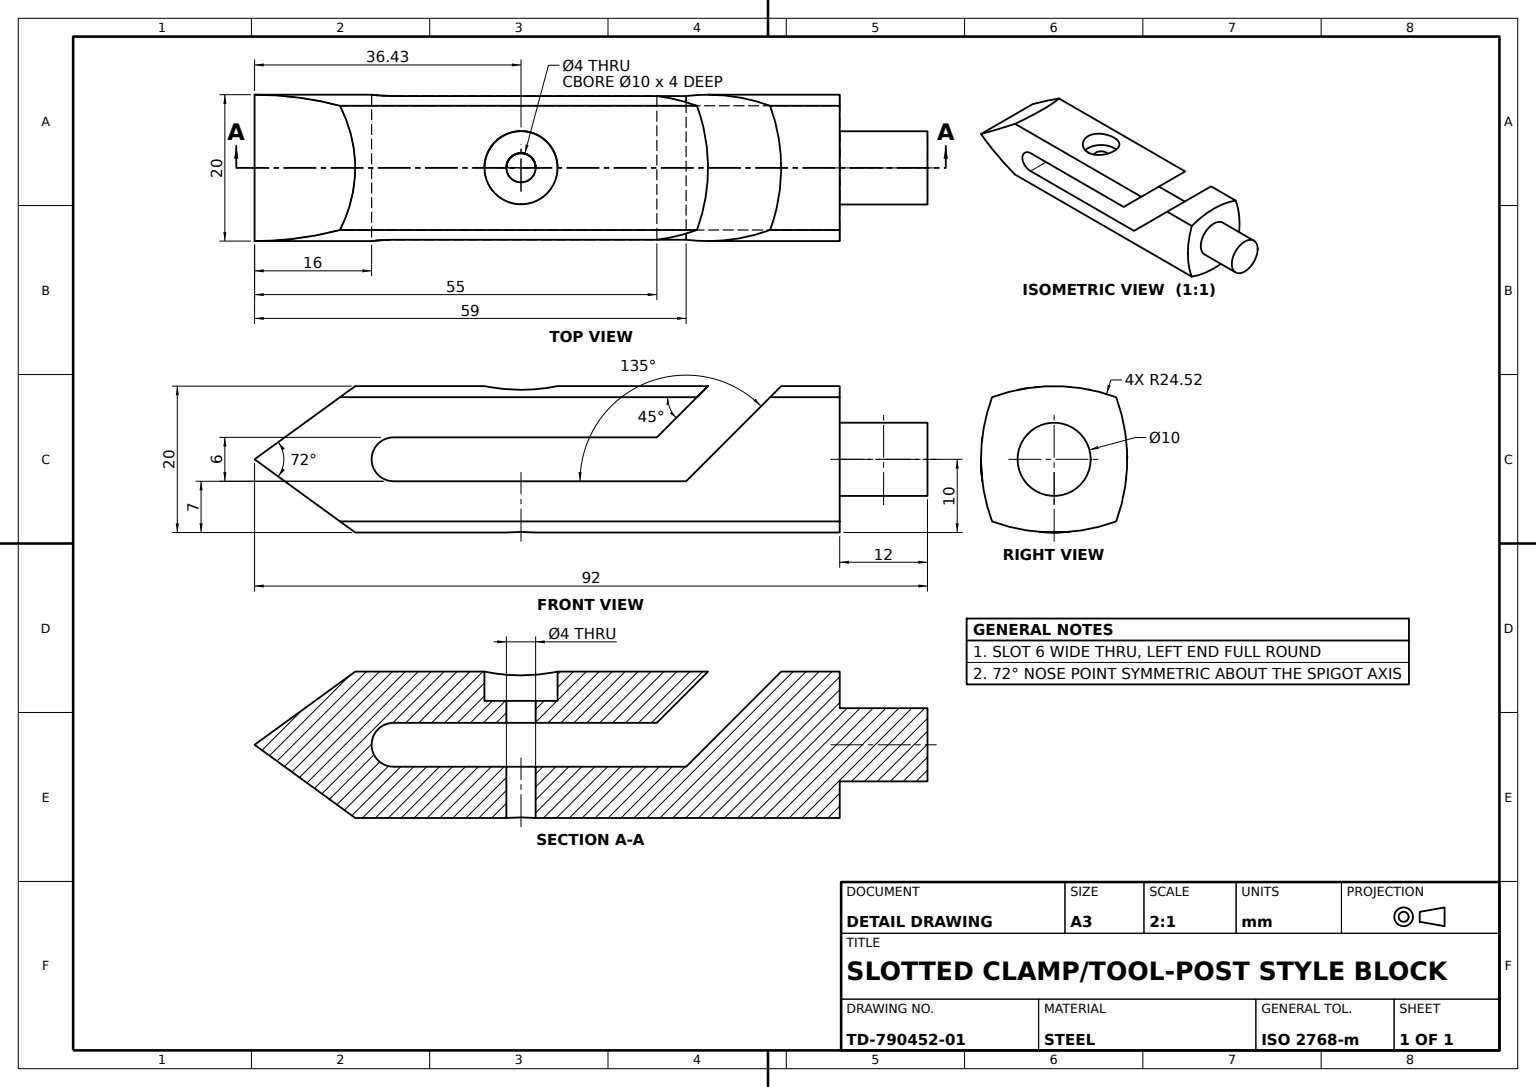
from build123d import *

# Parameters (mm, degrees)
PIN_BODY_80MM_DEPTH             = 80
ARROW_NOSE_CUT_DEPTH            = 82.240384046
ARROW_NOSE_CUT_DEPTH_BACK       = 82.240384046
SLOT_AND_STEP_CUT_DEPTH         = 82.240384046
SLOT_AND_STEP_CUT_DEPTH_BACK    = 82.240384046
SPIGOT_PROFILE_10_R             = 5
SPIGOT_10X12_DEPTH              = 12
COUNTERBORED_HOLE_4_D           = 4
COUNTERBORED_HOLE_4_DEPTH       = 100
COUNTERBORED_HOLE_4_CBORE_D     = 10
COUNTERBORED_HOLE_4_CBORE_DEPTH = 4


with BuildPart() as part:
    # Pin Body Profile → Pin Body 80mm (new body)
    with BuildSketch(Plane(origin=(0, 0, 0), x_dir=(0, 0, -1), z_dir=(1, 0, 0))):
        with BuildLine():
            ThreePointArc((-8.485281374, -8.485281374), (-10, 0), (-8.485281374, 8.485281374))
            ThreePointArc((-8.485281374, 8.485281374), (0, 10), (8.485281374, 8.485281374))
            ThreePointArc((8.485281374, 8.485281374), (10, 0), (8.485281374, -8.485281374))
            ThreePointArc((8.485281374, -8.485281374), (0, -10), (-8.485281374, -8.485281374))
        make_face()
    extrude(amount=PIN_BODY_80MM_DEPTH)

    # Arrow Nose Profile 72deg → Arrow Nose Cut (cut, two sides: drawn at the far end of the back side and taken through both)
    with BuildSketch(Plane.XY.offset(-ARROW_NOSE_CUT_DEPTH_BACK)):
        Polygon((0, 10), (0, 0), (13.763819205, 10), align=None)
        Polygon((13.763819205, -10), (0, 0), (0, -10), align=None)
    extrude(amount=ARROW_NOSE_CUT_DEPTH + ARROW_NOSE_CUT_DEPTH_BACK, mode=Mode.SUBTRACT)

    # Slot and Step Profile → Slot and Step Cut (cut, two sides: drawn at the far end of the back side and taken through both)
    with BuildSketch(Plane.XY.offset(-SLOT_AND_STEP_CUT_DEPTH_BACK)):
        with BuildLine():
            Line((72, 10), (59, -3))
            Line((59, -3), (19, -3))
            ThreePointArc((19, -3), (16, 0), (19, 3))
            Line((19, 3), (55, 3))
            Line((55, 3), (62, 10))
            Line((62, 10), (72, 10))
        make_face()
    extrude(amount=SLOT_AND_STEP_CUT_DEPTH + SLOT_AND_STEP_CUT_DEPTH_BACK, mode=Mode.SUBTRACT)

    # Spigot Profile Ø10 → Spigot Ø10x12 (add)
    with BuildSketch(Plane(origin=(80, 0, 0), x_dir=(0, 0, -1), z_dir=(1, 0, 0))):
        Circle(SPIGOT_PROFILE_10_R)
    extrude(amount=SPIGOT_10X12_DEPTH)

    # Counterbored Hole Ø4
    with Locations(Plane(origin=(36.427461815, 9.999980768, -0.030712762), x_dir=(0, 0.001252347692, 0.999999215812), z_dir=(0, 0.999999215812, -0.001252347692))):
        with Locations((0, 0)):
            CounterBoreHole(COUNTERBORED_HOLE_4_D / 2, COUNTERBORED_HOLE_4_CBORE_D / 2, COUNTERBORED_HOLE_4_CBORE_DEPTH, depth=COUNTERBORED_HOLE_4_DEPTH)


solid = part.part
